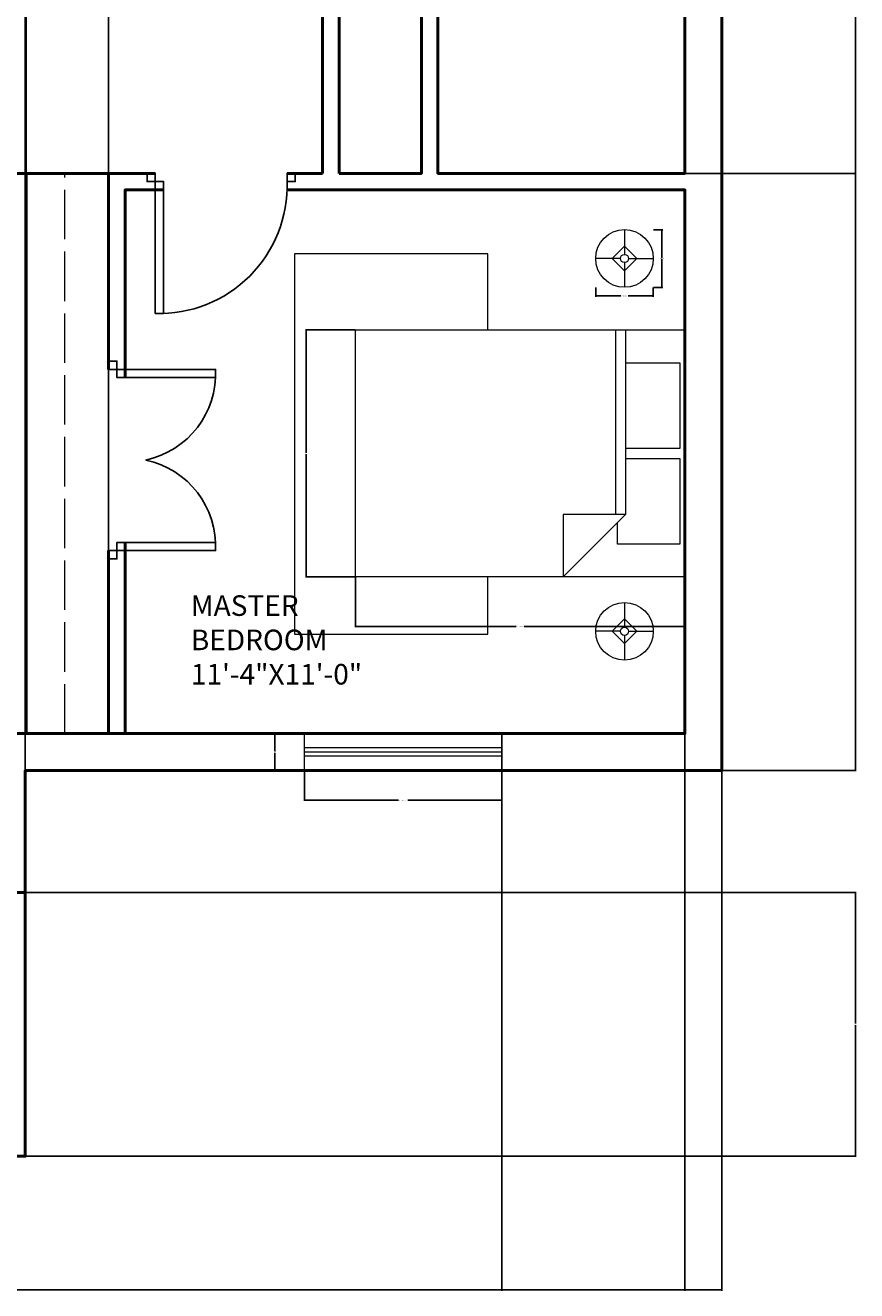
# Model space of a CAD drawing. Units: inches. Extents: x 821 to 2399, y 74 to 823.
# Tile 2 of 13: x 1128 to 1330, y 74 to 381. Entities that reach past the tile are written whole.
import ezdxf

# ---------------------------------------------------------------- set-up
doc = ezdxf.new("R2010")
doc.units = ezdxf.units.IN
doc.header["$MEASUREMENT"] = 0
doc.linetypes.add('ACAD_ISO02W100', pattern=[15, 12, -3])
doc.layers.get('0').update_dxf_attribs({"lineweight": 53})
for name, color, linetype, lineweight in [('A-ANNO-DIMS', 2, 'Continuous', 18), ('A-AREA-IDEN', 7, 'Continuous', 18), ('A-DOOR', 4, 'Continuous', 25), ('A-FURN', 8, 'Continuous', 18), ('A-GLAZ', 4, 'Continuous', 18), ('A-WALL-OVHD', 8, 'ACAD_ISO02W100', 18), ('WALLS', 7, 'Continuous', 50)]:
    doc.layers.add(name, color=color, linetype=linetype, lineweight=lineweight)
doc.styles.get("Standard").update_dxf_attribs({"font": 'arial.ttf'})
doc.dimstyles.get("Standard").update_dxf_attribs({"dimtxt": 0.18, "dimasz": 0.18, "dimexe": 0.18, "dimexo": 0.0625, "dimgap": 0.09, "dimtad": 0, "dimtih": 1, "dimtoh": 1, "dimdec": 4, "dimzin": 0, "dimdsep": 46, "dimtxsty": 'Standard', "dimcen": 0.09, "dimadec": 0, "dimazin": 0, "dimtfac": 1, "dimtdec": 4, "dimtofl": 0, "dimtmove": 0, "dimatfit": 3, "dimfxl": 1, "dimtolj": 1, "dimtzin": 0, "dimarcsym": 0})

# ---------------------------------------------------------------- blocks, each defined once
blk = doc.blocks.new('Bed - Queen')
for p, q in [((0, -80.00003), (0, 0)), ((0, 0), (59.99999, 0)), ((59.99999, 0), (59.99999, -80.00003)), ((7.99999, -1.2), (28.79998, -1.2)), ((7.99999, -14.4), (7.99999, -1.2)), ((28.79998, -1.2), (28.79998, -14.4)), ((31.19999, -1.2), (51.99999, -1.2)), ((31.19999, -14.4), (31.19999, -1.2)), ((51.99999, -1.2), (51.99999, -16.4)), ((0, -14.4), (44.8, -14.4)), ((59.99999, -29.6), (44.8, -14.4)), ((44.8, -14.4), (44.8, -29.6)), ((44.8, -16.8), (0, -16.8)), ((51.99999, -16.4), (46.79936, -16.4)), ((44.8, -29.6), (59.99999, -29.6)), ((59.99999, -80.00003), (0, -80.00003))]:
    blk.add_line(p, q)
blk = doc.blocks.new('Lamp - Table')
for p, q in [((0, 7), (0, 1)), ((-1, 0), (-7, 0)), ((0, 3), (-3, 0)), ((-3, 0), (0, -3)), ((3, 0), (0, 3)), ((0, -3), (3, 0)), ((1, 0), (7, 0)), ((0, -1), (0, -7))]:
    blk.add_line(p, q)
for radius in [7, 1]:
    blk.add_circle((0, 0), radius)
blk = doc.blocks.new('DOOR-SWING-32IN')
for p, q in [((0, 0), (2, 0)), ((34, 0), (36, 0))]:
    blk.add_line(p, q)
blk.add_lwpolyline([(34, 2, 0.433232), (2, 34), (4, 34), (4, 2), (2, 2), (2, 34)], format="xyb")
for points in [[(0, 0), (2, 0), (2, 2), (0, 2)], [(36, 0), (34, 0), (34, 2), (36, 2)]]:
    blk.add_lwpolyline(points, close=True)
blk = doc.blocks.new('WIN-48IN')
for p, q in [((3.5, 48), (3.5, 0)), ((4.5, 48), (4.5, 0)), ((5.5, 48), (5.5, 0))]:
    blk.add_line(p, q)
blk.add_lwpolyline([(9, 0), (0, 0), (0, 48), (9, 48)], close=True)
blk = doc.blocks.new('*D30')
at = {"layer": 'A-ANNO-DIMS', "color": 0, "lineweight": -2, "transparency": 16777216}
for p, q in [((1195.94, 200.46), (1195.94, 193.14)), ((1243.94, 200.46), (1243.94, 193.14)), ((1196.12, 193.32), (1218.83, 193.32)), ((1243.76, 193.32), (1221.06, 193.32))]:
    blk.add_line(p, q, dxfattribs=at)
at = {"layer": 'A-ANNO-DIMS', "color": 0, "lineweight": 50, "transparency": 16777216}
for points in [[(1196.12, 193.35), (1196.12, 193.29), (1195.94, 193.32)], [(1243.76, 193.35), (1243.76, 193.29), (1243.94, 193.32)]]:
    blk.add_solid(points, dxfattribs=at)
at = {"layer": 'Defpoints', "color": 0, "lineweight": 50, "transparency": 16777216}
for p in [(1195.94, 200.52), (1243.94, 200.52), (1243.94, 193.32)]:
    blk.add_point(p, dxfattribs=at)
at = {"layer": 'A-ANNO-DIMS', "color": 0, "transparency": 16777216, "insert": (1219.94, 193.32), "char_height": 0.18, "attachment_point": 5}
blk.add_mtext('\\A1;WINDOW 48 TYP.', dxfattribs=at)
blk = doc.blocks.new('*D31')
at = {"layer": 'A-ANNO-DIMS', "color": 0, "lineweight": -2, "transparency": 16777216}
for p, q in [((1195.88, 209.52), (1188.56, 209.52)), ((1188.74, 209.34), (1188.74, 205.2)), ((1188.74, 200.7), (1188.74, 204.84)), ((1195.88, 200.52), (1188.56, 200.52))]:
    blk.add_line(p, q, dxfattribs=at)
at = {"layer": 'A-ANNO-DIMS', "color": 0, "lineweight": 50, "transparency": 16777216}
for points in [[(1188.71, 209.34), (1188.77, 209.34), (1188.74, 209.52)], [(1188.71, 200.7), (1188.77, 200.7), (1188.74, 200.52)]]:
    blk.add_solid(points, dxfattribs=at)
at = {"layer": 'Defpoints', "color": 0, "lineweight": 50, "transparency": 16777216}
for p in [(1195.94, 209.52), (1188.74, 200.52), (1195.94, 200.52)]:
    blk.add_point(p, dxfattribs=at)
at = {"layer": 'A-ANNO-DIMS', "color": 0, "transparency": 16777216, "insert": (1188.74, 205.02), "char_height": 0.18, "attachment_point": 5}
blk.add_mtext('\\A1;9 TYP.', dxfattribs=at)
blk = doc.blocks.new('*D34')
at = {"layer": 'A-ANNO-DIMS', "color": 0, "lineweight": -2, "transparency": 16777216}
for p, q in [((1266.71, 317.79), (1266.71, 315.57)), ((1280.71, 317.79), (1280.71, 315.57)), ((1266.89, 315.75), (1272.81, 315.75)), ((1280.53, 315.75), (1274.61, 315.75))]:
    blk.add_line(p, q, dxfattribs=at)
at = {"layer": 'A-ANNO-DIMS', "color": 0, "lineweight": 50, "transparency": 16777216}
for points in [[(1266.89, 315.78), (1266.89, 315.72), (1266.71, 315.75)], [(1280.53, 315.78), (1280.53, 315.72), (1280.71, 315.75)]]:
    blk.add_solid(points, dxfattribs=at)
at = {"layer": 'Defpoints', "color": 0, "lineweight": 50, "transparency": 16777216}
for p in [(1266.71, 317.85), (1280.71, 317.85), (1280.71, 315.75)]:
    blk.add_point(p, dxfattribs=at)
at = {"layer": 'A-ANNO-DIMS', "color": 0, "transparency": 16777216, "insert": (1273.71, 315.75), "char_height": 0.18, "attachment_point": 5}
blk.add_mtext('\\A1;LAMP 14 TYP.', dxfattribs=at)
blk = doc.blocks.new('*D35')
at = {"layer": 'A-ANNO-DIMS', "color": 0, "lineweight": -2, "transparency": 16777216}
for p, q in [((1280.77, 331.85), (1282.99, 331.85)), ((1282.81, 331.67), (1282.81, 325.03)), ((1282.81, 318.03), (1282.81, 324.67)), ((1280.77, 317.85), (1282.99, 317.85))]:
    blk.add_line(p, q, dxfattribs=at)
at = {"layer": 'A-ANNO-DIMS', "color": 0, "lineweight": 50, "transparency": 16777216}
for points in [[(1282.78, 331.67), (1282.84, 331.67), (1282.81, 331.85)], [(1282.78, 318.03), (1282.84, 318.03), (1282.81, 317.85)]]:
    blk.add_solid(points, dxfattribs=at)
at = {"layer": 'Defpoints', "color": 0, "lineweight": 50, "transparency": 16777216}
for p in [(1280.71, 331.85), (1282.81, 331.85), (1280.71, 317.85)]:
    blk.add_point(p, dxfattribs=at)
at = {"layer": 'A-ANNO-DIMS', "color": 0, "transparency": 16777216, "insert": (1282.81, 324.85), "char_height": 0.18, "attachment_point": 5}
blk.add_mtext('\\A1;14 TYP.', dxfattribs=at)
blk = doc.blocks.new('*D44')
at = {"layer": 'A-ANNO-DIMS', "color": 0, "lineweight": -2, "transparency": 16777216}
for p, q in [((1208.37, 247.46), (1208.37, 235.34)), ((1288.37, 247.46), (1288.37, 235.34)), ((1208.55, 235.52), (1247.38, 235.52)), ((1288.19, 235.52), (1249.37, 235.52))]:
    blk.add_line(p, q, dxfattribs=at)
at = {"layer": 'A-ANNO-DIMS', "color": 0, "lineweight": 50, "transparency": 16777216}
for points in [[(1208.55, 235.55), (1208.55, 235.49), (1208.37, 235.52)], [(1288.19, 235.55), (1288.19, 235.49), (1288.37, 235.52)]]:
    blk.add_solid(points, dxfattribs=at)
at = {"layer": 'Defpoints', "color": 0, "lineweight": 50, "transparency": 16777216}
for p in [(1208.37, 247.52), (1288.37, 247.52), (1288.37, 235.52)]:
    blk.add_point(p, dxfattribs=at)
at = {"layer": 'A-ANNO-DIMS', "color": 0, "transparency": 16777216, "insert": (1248.37, 235.52), "char_height": 0.18, "attachment_point": 5}
blk.add_mtext('\\A1;QUEEN BED 80', dxfattribs=at)
blk = doc.blocks.new('*D45')
at = {"layer": 'A-ANNO-DIMS', "color": 0, "lineweight": -2, "transparency": 16777216}
for p, q in [((1208.31, 307.52), (1196.19, 307.52)), ((1196.37, 307.34), (1196.37, 277.7)), ((1196.37, 247.7), (1196.37, 277.34)), ((1208.31, 247.52), (1196.19, 247.52))]:
    blk.add_line(p, q, dxfattribs=at)
at = {"layer": 'A-ANNO-DIMS', "color": 0, "lineweight": 50, "transparency": 16777216}
for points in [[(1196.34, 307.34), (1196.4, 307.34), (1196.37, 307.52)], [(1196.34, 247.7), (1196.4, 247.7), (1196.37, 247.52)]]:
    blk.add_solid(points, dxfattribs=at)
at = {"layer": 'Defpoints', "color": 0, "lineweight": 50, "transparency": 16777216}
for p in [(1208.37, 307.52), (1196.37, 247.52), (1208.37, 247.52)]:
    blk.add_point(p, dxfattribs=at)
at = {"layer": 'A-ANNO-DIMS', "color": 0, "transparency": 16777216, "insert": (1196.37, 277.52), "char_height": 0.18, "attachment_point": 5}
blk.add_mtext('\\A1;60', dxfattribs=at)
blk = doc.blocks.new('*D78')
at = {"layer": 'A-ANNO-DIMS', "color": 0, "lineweight": -2, "transparency": 16777216}
for p, q in [((853.37, 292.49), (853.37, 74.23)), ((1297.37, 200.46), (1297.37, 74.23)), ((853.55, 74.41), (1075.08, 74.41)), ((1297.19, 74.41), (1075.67, 74.41))]:
    blk.add_line(p, q, dxfattribs=at)
at = {"layer": 'A-ANNO-DIMS', "color": 0, "lineweight": 50, "transparency": 16777216}
for points in [[(853.55, 74.44), (853.55, 74.38), (853.37, 74.41)], [(1297.19, 74.44), (1297.19, 74.38), (1297.37, 74.41)]]:
    blk.add_solid(points, dxfattribs=at)
at = {"layer": 'Defpoints', "color": 0, "lineweight": 50, "transparency": 16777216}
for p in [(853.37, 292.55), (1297.37, 200.52), (1297.37, 74.41)]:
    blk.add_point(p, dxfattribs=at)
at = {"layer": 'A-ANNO-DIMS', "color": 0, "transparency": 16777216, "insert": (1075.37, 74.41), "char_height": 0.18, "attachment_point": 5}
blk.add_mtext('\\A1;444', dxfattribs=at)
blk = doc.blocks.new('*D79')
at = {"layer": 'A-ANNO-DIMS', "color": 0, "lineweight": -2, "transparency": 16777216}
for p, q in [((1297.44, 598.52), (1330, 598.52)), ((1329.82, 598.34), (1329.82, 399.7)), ((1329.82, 200.7), (1329.82, 399.34)), ((1297.44, 200.52), (1330, 200.52))]:
    blk.add_line(p, q, dxfattribs=at)
at = {"layer": 'A-ANNO-DIMS', "color": 0, "lineweight": 50, "transparency": 16777216}
for points in [[(1329.79, 598.34), (1329.85, 598.34), (1329.82, 598.52)], [(1329.79, 200.7), (1329.85, 200.7), (1329.82, 200.52)]]:
    blk.add_solid(points, dxfattribs=at)
at = {"layer": 'Defpoints', "color": 0, "lineweight": 50, "transparency": 16777216}
for p in [(1297.37, 598.52), (1297.37, 200.52), (1329.82, 200.52)]:
    blk.add_point(p, dxfattribs=at)
at = {"layer": 'A-ANNO-DIMS', "color": 0, "transparency": 16777216, "insert": (1329.82, 399.52), "char_height": 0.18, "attachment_point": 5}
blk.add_mtext('\\A1;398', dxfattribs=at)
blk = doc.blocks.new('*D88')
at = {"layer": 'A-ANNO-DIMS', "color": 0, "lineweight": -2, "transparency": 16777216}
for p, q in [((1128.19, 170.94), (1330, 170.94)), ((1329.82, 170.76), (1329.82, 139.08)), ((1329.82, 107.04), (1329.82, 138.72)), ((1128.19, 106.86), (1330, 106.86))]:
    blk.add_line(p, q, dxfattribs=at)
at = {"layer": 'A-ANNO-DIMS', "color": 0, "lineweight": 50, "transparency": 16777216}
for points in [[(1329.79, 170.76), (1329.85, 170.76), (1329.82, 170.94)], [(1329.79, 107.04), (1329.85, 107.04), (1329.82, 106.86)]]:
    blk.add_solid(points, dxfattribs=at)
at = {"layer": 'Defpoints', "color": 0, "lineweight": 50, "transparency": 16777216}
for p in [(1128.12, 170.94), (1128.12, 106.86), (1329.82, 106.86)]:
    blk.add_point(p, dxfattribs=at)
at = {"layer": 'A-ANNO-DIMS', "color": 0, "transparency": 16777216, "insert": (1329.82, 138.9), "char_height": 0.18, "attachment_point": 5}
blk.add_mtext('\\A1;64.08', dxfattribs=at)
blk = doc.blocks.new('*D89')
at = {"layer": 'A-ANNO-DIMS', "color": 0, "lineweight": -2, "transparency": 16777216}
for p, q in [((1050.64, 106.93), (1050.64, 786.75)), ((1050.82, 786.57), (1088.99, 786.57)), ((1127.94, 786.57), (1089.78, 786.57)), ((1128.12, 106.93), (1128.12, 786.75))]:
    blk.add_line(p, q, dxfattribs=at)
at = {"layer": 'A-ANNO-DIMS', "color": 0, "lineweight": 50, "transparency": 16777216}
for points in [[(1050.82, 786.6), (1050.82, 786.54), (1050.64, 786.57)], [(1127.94, 786.6), (1127.94, 786.54), (1128.12, 786.57)]]:
    blk.add_solid(points, dxfattribs=at)
at = {"layer": 'Defpoints', "color": 0, "lineweight": 50, "transparency": 16777216}
for p in [(1128.12, 786.57), (1050.64, 106.86), (1128.12, 106.86)]:
    blk.add_point(p, dxfattribs=at)
at = {"layer": 'A-ANNO-DIMS', "color": 0, "transparency": 16777216, "insert": (1089.38, 786.57), "char_height": 0.18, "attachment_point": 5}
blk.add_mtext('\\A1;77.48', dxfattribs=at)
blk = doc.blocks.new('*D92')
at = {"layer": 'A-ANNO-DIMS', "color": 0, "lineweight": -2, "transparency": 16777216}
for p, q in [((1128.37, 209.58), (1128.37, 786.75)), ((1128.55, 786.57), (1138.15, 786.57)), ((1148.19, 786.57), (1138.59, 786.57)), ((1148.37, 209.58), (1148.37, 786.75))]:
    blk.add_line(p, q, dxfattribs=at)
at = {"layer": 'A-ANNO-DIMS', "color": 0, "lineweight": 50, "transparency": 16777216}
for points in [[(1128.55, 786.6), (1128.55, 786.54), (1128.37, 786.57)], [(1148.19, 786.6), (1148.19, 786.54), (1148.37, 786.57)]]:
    blk.add_solid(points, dxfattribs=at)
at = {"layer": 'Defpoints', "color": 0, "lineweight": 50, "transparency": 16777216}
for p in [(1148.37, 786.57), (1128.37, 209.52), (1148.37, 209.52)]:
    blk.add_point(p, dxfattribs=at)
at = {"layer": 'A-ANNO-DIMS', "color": 0, "transparency": 16777216, "insert": (1138.37, 786.57), "char_height": 0.18, "attachment_point": 5}
blk.add_mtext('\\A1;20', dxfattribs=at)
blk = doc.blocks.new('*D93')
at = {"layer": 'A-ANNO-DIMS', "color": 0, "lineweight": -2, "transparency": 16777216}
for p, q in [((1243.94, 209.46), (1243.94, 74.23)), ((1288.37, 209.46), (1288.37, 74.23)), ((1244.12, 74.41), (1265.76, 74.41)), ((1288.19, 74.41), (1266.56, 74.41))]:
    blk.add_line(p, q, dxfattribs=at)
at = {"layer": 'A-ANNO-DIMS', "color": 0, "lineweight": 50, "transparency": 16777216}
for points in [[(1244.12, 74.44), (1244.12, 74.38), (1243.94, 74.41)], [(1288.19, 74.44), (1288.19, 74.38), (1288.37, 74.41)]]:
    blk.add_solid(points, dxfattribs=at)
at = {"layer": 'Defpoints', "color": 0, "lineweight": 50, "transparency": 16777216}
for p in [(1243.94, 209.52), (1288.37, 209.52), (1243.94, 74.41)]:
    blk.add_point(p, dxfattribs=at)
at = {"layer": 'A-ANNO-DIMS', "color": 0, "transparency": 16777216, "insert": (1266.16, 74.41), "char_height": 0.18, "attachment_point": 5}
blk.add_mtext('\\A1;44.43', dxfattribs=at)
blk = doc.blocks.new('*D96')
at = {"layer": 'A-ANNO-DIMS', "color": 0, "lineweight": -2, "transparency": 16777216}
for p, q in [((1288.44, 396.52), (1330, 396.52)), ((1329.82, 396.34), (1329.82, 371.2)), ((1329.82, 345.7), (1329.82, 370.84)), ((1288.44, 345.52), (1330, 345.52))]:
    blk.add_line(p, q, dxfattribs=at)
at = {"layer": 'A-ANNO-DIMS', "color": 0, "lineweight": 50, "transparency": 16777216}
for points in [[(1329.79, 396.34), (1329.85, 396.34), (1329.82, 396.52)], [(1329.79, 345.7), (1329.85, 345.7), (1329.82, 345.52)]]:
    blk.add_solid(points, dxfattribs=at)
at = {"layer": 'Defpoints', "color": 0, "lineweight": 50, "transparency": 16777216}
for p in [(1288.37, 396.52), (1288.37, 345.52), (1329.82, 345.52)]:
    blk.add_point(p, dxfattribs=at)
at = {"layer": 'A-ANNO-DIMS', "color": 0, "transparency": 16777216, "insert": (1329.82, 371.02), "char_height": 0.18, "attachment_point": 5}
blk.add_mtext('\\A1;51', dxfattribs=at)

msp = doc.modelspace()

# ---------------------------------------------------------------- linework, layer by layer
at = {"layer": 'A-DOOR'}
for points in [[(1148.3735, 299.9247), (1150.3735, 299.9247), (1150.3735, 297.9247), (1148.3735, 297.9247)], [(1148.3735, 251.9247), (1150.3735, 251.9247), (1150.3735, 253.9247), (1148.3735, 253.9247)]]:
    msp.add_lwpolyline(points, close=True, dxfattribs=at)
msp.add_lwpolyline([(1174.3735, 297.9247), (1174.3735, 295.9247), (1150.3735, 295.9247), (1150.3735, 297.9247), (1174.3735, 297.9247, -0.36630785), (1157.4504, 275.9247, -0.36630785), (1174.3735, 253.9247), (1150.3735, 253.9247), (1150.3735, 255.9247), (1174.3735, 255.9247), (1174.3735, 253.9247)], format="xyb", dxfattribs=at)
at = {"layer": 'A-FURN'}
msp.add_lwpolyline([(1240.5391, 307.5195), (1240.5391, 325.9641), (1193.534, 325.9641), (1193.534, 233.6283), (1240.5391, 233.6283), (1240.5391, 247.5195)], dxfattribs=at)
at = {"layer": 'A-WALL-OVHD'}
msp.add_line((1137.7279, 209.5195), (1137.7279, 345.5195), dxfattribs=at)
at = {"layer": 'WALLS'}
for p, q in [((1200.3735, 345.5195), (1200.3735, 396.5195)), ((1124.3735, 345.5195), (1159.7172, 345.5195)), ((1191.7172, 345.5195), (1200.3735, 345.5195)), ((1288.3735, 307.5195), (1288.3735, 209.5195)), ((1152.3735, 209.5195), (1152.3735, 255.9247)), ((1148.3735, 209.5195), (1148.3735, 253.9247))]:
    msp.add_line(p, q, dxfattribs=at)
for points in [[(1050.641, 200.5195), (1050.641, 170.9407), (1121.9086, 170.9407), (1128.124, 170.9407), (1050.641, 170.9407), (1050.641, 106.8645), (1128.124, 106.8645), (1128.124, 170.9407), (1128.124, 200.5195), (1288.3735, 200.5195), (1297.3735, 200.5195), (1297.3735, 598.5195), (853.3735, 598.5195), (853.3735, 292.549), (922.3673, 292.5195), (1043.3735, 292.5195), (1043.3735, 209.5195), (1043.3735, 200.5195)], [(1204.3735, 345.5195), (1204.3735, 396.5195), (1224.3735, 396.5195), (1224.3735, 345.5195)], [(1288.3735, 396.5195), (1228.3735, 396.5195), (1228.3735, 345.5195), (1288.3735, 345.5195)]]:
    msp.add_lwpolyline(points, close=True, dxfattribs=at)
for points in [[(1128.3735, 209.5195), (1128.3735, 341.5195), (1128.3735, 345.5195)], [(1148.3735, 297.9247), (1148.3735, 341.5195), (1148.3735, 345.5195)], [(1191.7172, 341.5195), (1288.3735, 341.5195), (1288.3735, 209.5195), (1103.5667, 209.5195)], [(1152.3735, 295.9247), (1152.3735, 341.5195), (1161.7172, 341.5195)]]:
    msp.add_lwpolyline(points, dxfattribs=at)

# ---------------------------------------------------------------- block references
at = {"layer": 'A-DOOR', "extrusion": (0, 0, -1), "zscale": -1, "rotation": 180}
msp.add_blockref('DOOR-SWING-32IN', (-1157.7168, 345.5199), dxfattribs=at)
at = {"layer": 'A-FURN'}
for p in [(1273.7076, 324.8524), (1273.7076, 234.3347)]:
    msp.add_blockref('Lamp - Table', p, dxfattribs=at)
at = {"layer": 'A-FURN', "rotation": 270}
msp.add_blockref('Bed - Queen', (1288.3735, 307.5195), dxfattribs=at)
at = {"layer": 'A-GLAZ', "rotation": 269.9999999999985}
msp.add_blockref('WIN-48IN', (1195.9438, 209.5199), dxfattribs=at)

# ---------------------------------------------------------------- texts
at = {"layer": 'A-AREA-IDEN', "insert": (1168.3509, 243.0804), "char_height": 5, "attachment_point": 1}
msp.add_mtext_dynamic_manual_height_columns('MASTER\\PBEDROOM\\P11\'-4"X11\'-0"', width=59.754275, gutter_width=1, heights=[0], dxfattribs=at)

# ---------------------------------------------------------------- dimensions: what is measured, and where the dimension line sits
at = {"layer": 'A-ANNO-DIMS'}
for base, p1, p2, override, picture, middle in [((1128.124, 786.5664), (1050.641, 106.8645), (1128.124, 106.8645), {"dimdec": 2, "dimlfac": 1, "dimrnd": 0, "dimzin": 0, "dimdsep": 46, "dimlunit": 2}, '*D89', (1089.3825, 786.5664)), ((1148.3735, 786.5664), (1128.3735, 209.5195), (1148.3735, 209.5195), {"dimdec": 0, "dimlfac": 1, "dimrnd": 0, "dimzin": 0, "dimdsep": 46, "dimlunit": 2}, '*D92', (1138.3735, 786.5664)), ((1297.3735, 74.4145), (853.3735, 292.549), (1297.3735, 200.5195), {"dimdec": 0, "dimlfac": 1, "dimrnd": 0, "dimzin": 0, "dimdsep": 46, "dimlunit": 2}, '*D78', (1075.3735, 74.4145)), ((1243.944, 74.4145), (1288.3735, 209.5195), (1243.944, 209.5195), {"dimdec": 2, "dimlfac": 1, "dimrnd": 0, "dimzin": 0, "dimdsep": 46, "dimlunit": 2}, '*D93', (1266.1587, 74.4145))]:
    dim = msp.add_linear_dim(base=base, p1=p1, p2=p2, dimstyle='Standard', override=override, dxfattribs=at)
    dim.commit()
    dim.dimension.update_dxf_attribs({"geometry": picture, "text_midpoint": middle})
for base, p1, p2, angle, override, picture, middle in [((1329.8235, 200.5195), (1297.3735, 598.5195), (1297.3735, 200.5195), 90, {"dimdec": 0, "dimlfac": 1, "dimrnd": 0, "dimzin": 0, "dimdsep": 46, "dimlunit": 2}, '*D79', (1329.8235, 399.5195)), ((1329.8235, 345.5195), (1288.3735, 396.5195), (1288.3735, 345.5195), 90, {"dimdec": 0, "dimlfac": 1, "dimrnd": 0, "dimzin": 0, "dimdsep": 46, "dimlunit": 2}, '*D96', (1329.8235, 371.0195)), ((1196.3734, 247.5195), (1208.3734, 307.5195), (1208.3734, 247.5195), 270, {"dimdec": 0, "dimlfac": 1, "dimrnd": 0, "dimzin": 0, "dimdsep": 46, "dimlunit": 2}, '*D45', (1196.3734, 277.5195)), ((1329.8235, 106.8645), (1128.124, 170.9407), (1128.124, 106.8645), 90, {"dimdec": 2, "dimlfac": 1, "dimrnd": 0, "dimzin": 0, "dimdsep": 46, "dimlunit": 2}, '*D88', (1329.8235, 138.9026))]:
    dim = msp.add_linear_dim(base=base, p1=p1, p2=p2, angle=angle, dimstyle='Standard', override=override, dxfattribs=at)
    dim.commit()
    dim.dimension.update_dxf_attribs({"geometry": picture, "text_midpoint": middle})
for base, p1, p2, angle, picture, middle in [((1282.8076, 331.8524), (1280.7076, 317.8524), (1280.7076, 331.8524), 90, '*D35', (1282.8076, 324.8524)), ((1188.744, 200.5195), (1195.944, 209.5195), (1195.944, 200.5195), 270, '*D31', (1188.744, 205.0195))]:
    dim = msp.add_linear_dim(base=base, p1=p1, p2=p2, angle=angle, text='<> TYP.', dimstyle='Standard', override={"dimdec": 0, "dimlfac": 1, "dimrnd": 0, "dimzin": 0, "dimdsep": 46, "dimlunit": 2}, dxfattribs=at)
    dim.commit()
    dim.dimension.update_dxf_attribs({"geometry": picture, "text_midpoint": middle})
for base, p1, p2, text, picture, middle in [((1280.7076, 315.7524), (1266.7076, 317.8524), (1280.7076, 317.8524), 'LAMP <> TYP.', '*D34', (1273.7076, 315.7524)), ((1288.3735, 235.5195), (1208.3734, 247.5195), (1288.3735, 247.5195), 'QUEEN BED <>', '*D44', (1248.3734, 235.5195)), ((1243.944, 193.3195), (1195.944, 200.5195), (1243.944, 200.5195), 'WINDOW <> TYP.', '*D30', (1219.944, 193.3195))]:
    dim = msp.add_linear_dim(base=base, p1=p1, p2=p2, text=text, dimstyle='Standard', override={"dimdec": 0, "dimlfac": 1, "dimrnd": 0, "dimzin": 0, "dimdsep": 46, "dimlunit": 2}, dxfattribs=at)
    dim.commit()
    dim.dimension.update_dxf_attribs({"geometry": picture, "text_midpoint": middle})

doc.saveas('drawing.dxf')
